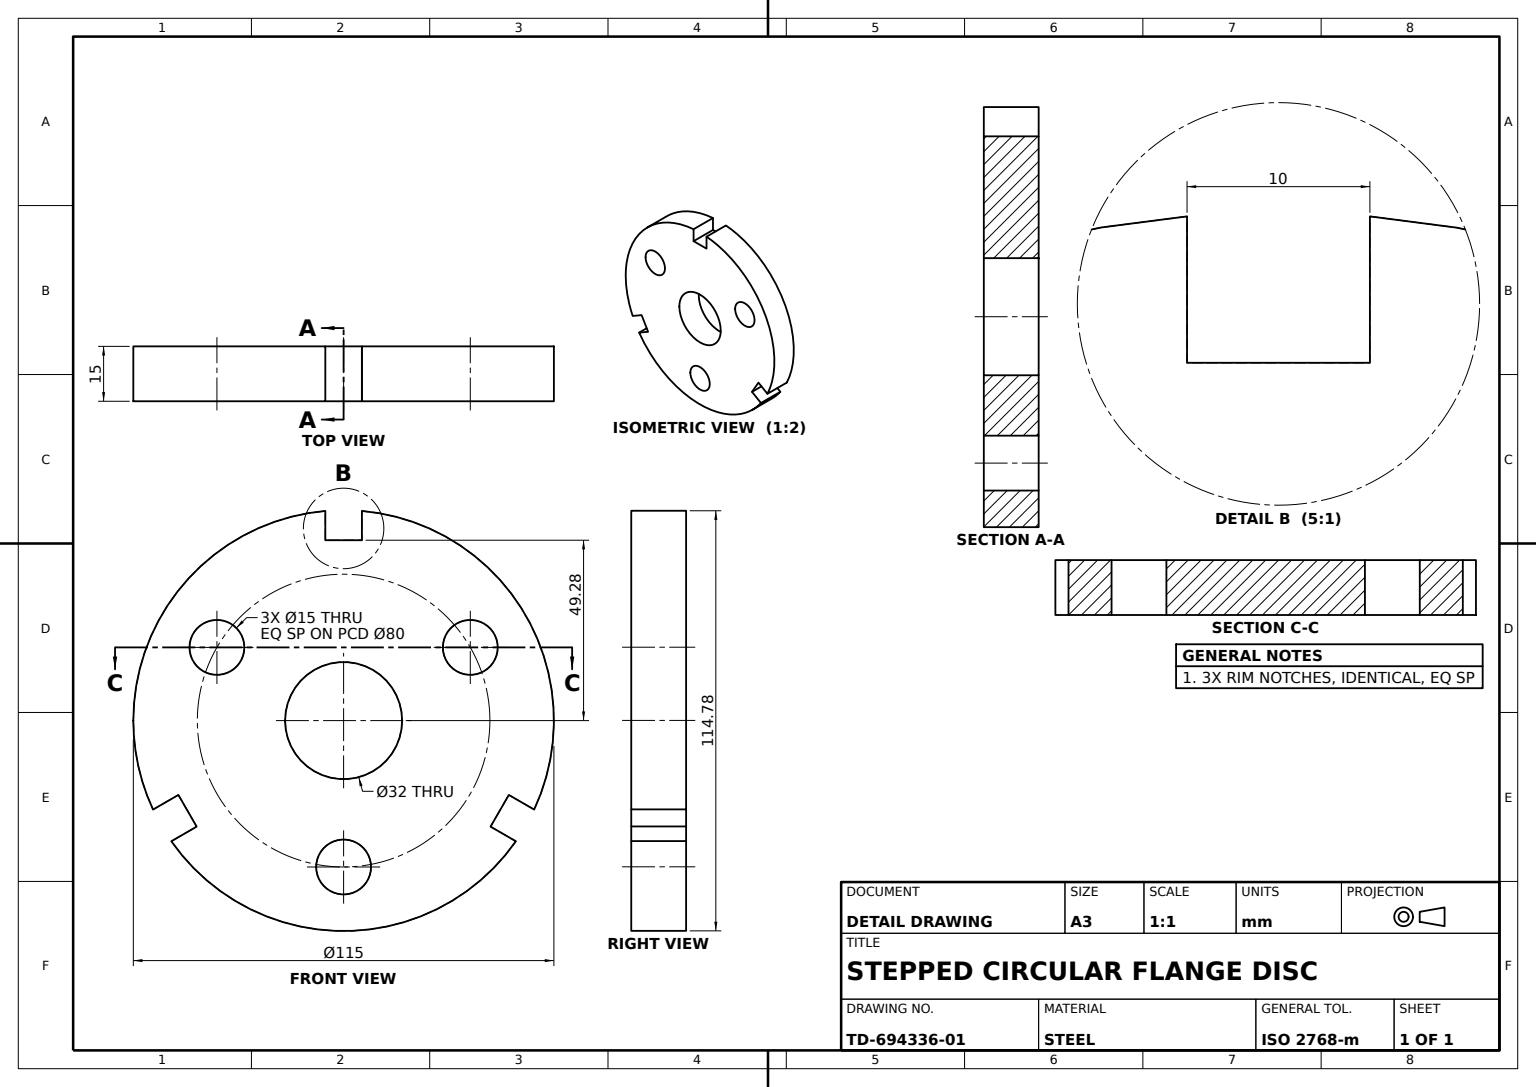
SolidWorks part; units mm, degrees
material "Plain Carbon Steel"
ref_plane "Front Plane" through (0, 0, 0) normal (0, 0, 1) x (1, 0, 0)
ref_plane "Top Plane" through (0, 0, 0) normal (0, 1, 0) x (1, 0, 0)
ref_plane "Right Plane" through (0, 0, 0) normal (1, 0, 0) x (0, 0, -1)
sketch "Disc Profile Ø115" plane through (0, 0, 0) normal (0, 0, 1) x (1, 0, 0)
  circle A0 centre (0, 0) radius 57.5
  dimension "D1" = 115
extrude "Disc Ø115x15" add sketch "Disc Profile Ø115" along normal blind 15
sketch "Holes 4xØ15 Sketch" plane through (0, 0, 15) normal (0, 0, 1) x (1, 0, 0)
  line L0 (0, 0) -> (57.5, 0)
  line L1 (0, 0) -> (34.641, 20)
  line L2 (0, 0) -> (0, -40)
  line L3 (0, 0) -> (-40, 0)
  line L4 (0, 0) -> (-34.641, 20)
  circle A0 centre (0, 0) radius 40
  circle A1 centre (0, 0) radius 57.5 construction
  circle A2 centre (34.641, 20) radius 7.5
  circle A3 centre (0, -40) radius 7.5
  circle A4 centre (-34.641, 20) radius 7.5
  dimension "D1" = 80
  dimension "D3" = 15
  dimension "D4" = 15
  dimension "D6" = 15
  dimension "D2" = 30
  dimension "D5" = 30
extrude "Holes 4xØ15 on Ø80" cut sketch "Holes 4xØ15 Sketch" against normal blind 15 contours A0 A4 | A0 A4 L4 | L4 A4 A0 | A0 A3 | L2 A3 A0 | A0 A3 L2 | A0 A2 | A0 A2 L1 | L1 A2 A0
sketch "Centre Bore Ø32 Sketch" plane through (0, 0, 15) normal (0, 0, 1) x (1, 0, 0)
  circle A0 centre (0, 0) radius 16
  dimension "D1" = 32
extrude "Centre Bore Ø32" cut sketch "Centre Bore Ø32 Sketch" against normal blind 15
sketch "Rim Notches Sketch" plane through (0, 0, 15) normal (0, 0, 1) x (1, 0, 0)
  line L0 (-5, 49.2822) -> (5, 49.2822)
  line L2 (-5, 49.2822) -> (-5, 57.2822)
  line L4 (5, 57.2822) -> (5, 49.2822)
  line L6 (45.1796, -20.311) -> (40.1796, -28.9712)
  line L7 (-40.1796, -28.9712) -> (-45.1796, -20.311)
  line L8 (45.1796, -20.311) -> (52.1078, -24.311)
  line L9 (-40.1796, -28.9712) -> (-47.1078, -32.9712)
  line L10 (47.1078, -32.9712) -> (40.1796, -28.9712)
  line L11 (-52.1078, -24.311) -> (-45.1796, -20.311)
  arc A0 (47.1078, -32.9712) -> (52.1078, -24.311) centre (0, 0) ccw
  arc A1 (5, 57.2822) -> (-5, 57.2822) centre (0, 0) ccw
  arc A2 (-52.1078, -24.311) -> (-47.1078, -32.9712) centre (0, 0) ccw
  point P2 (0, 49.2822)
  dimension "D1" = 3
  dimension "D2" = 3
  dimension "D3" = 3
  dimension "D4" = 3
  dimension "D5" = 10
  dimension "D6" = 8
  dimension "D7" = 49.2822
  dimension "D8" = 57.2822
  dimension "D9" = 40.1796
extrude "Rim Notches" cut sketch "Rim Notches Sketch" against normal blind 15
